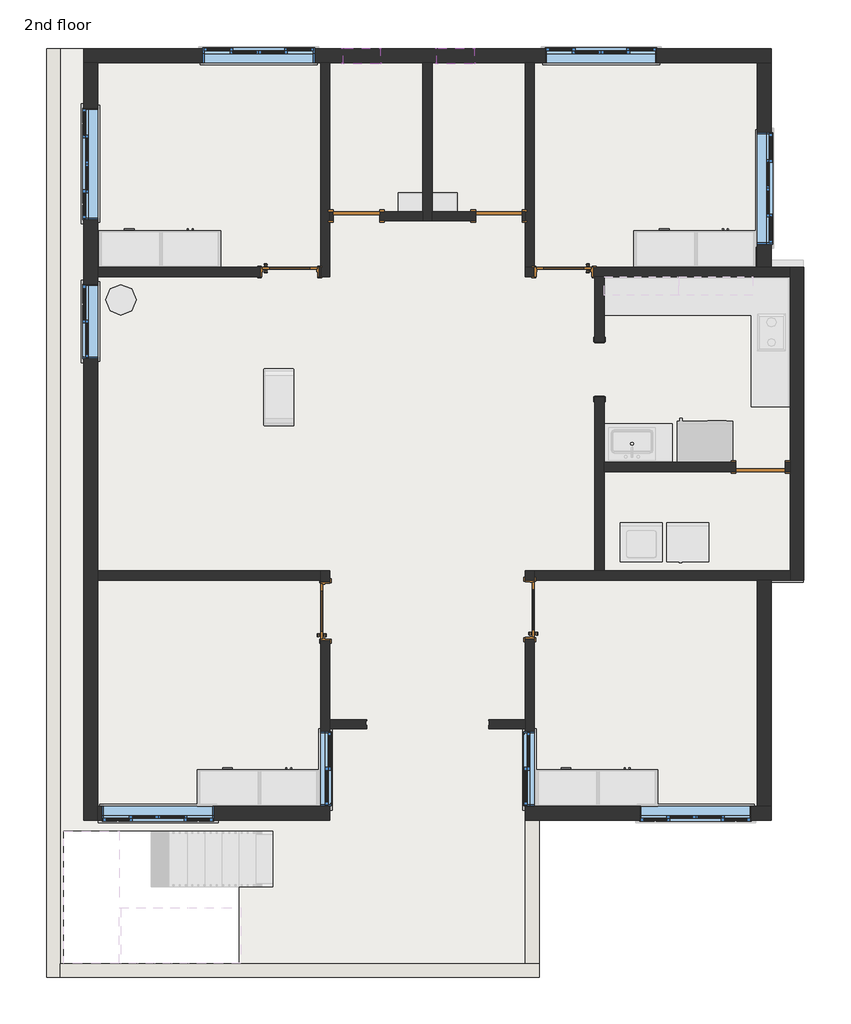
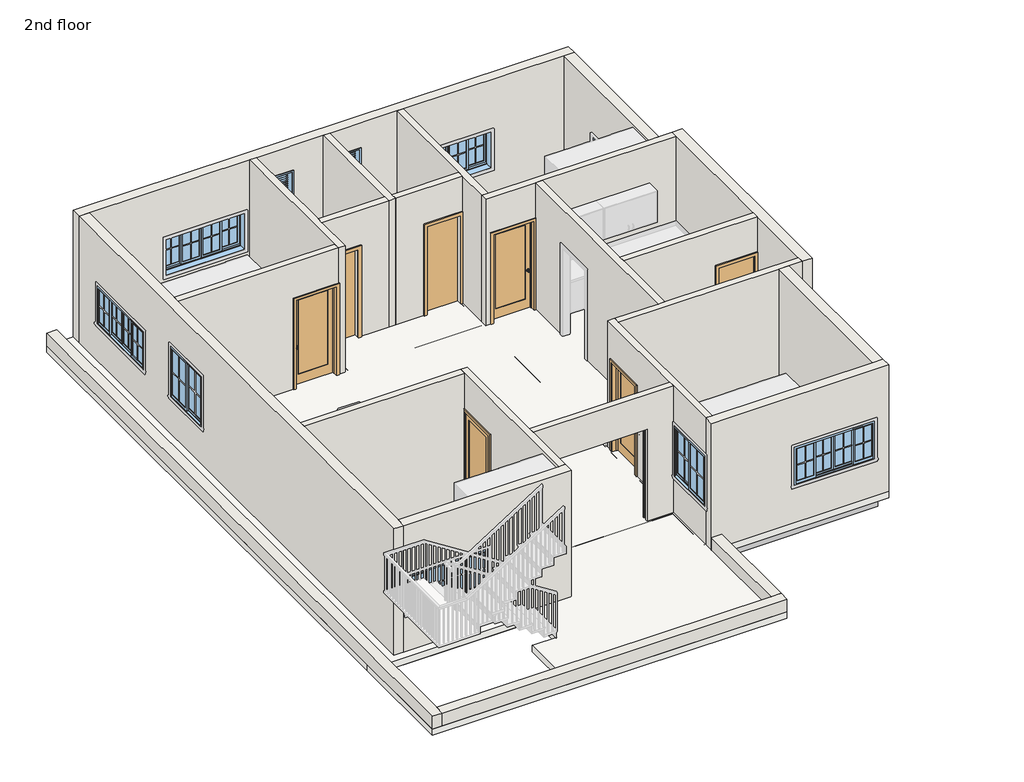
# One storey, part 1 of 4: 24 walls, 11 windows, 7 beams, 7 doors, 1 slab.
# Revit data of these elements (continued)
# Element 45 (IfcWindow, "Window-Sliding-Four : 72\" x 36\"") (continued)
#   Interior Wall Closure = 0' - 2 3/4"
#   Frame Extension = 0' - 0 1/4"
#   Exterior Wall Closure = 0' - 1 1/4"
#   Interior Trim Visibility = yes
#   Indicator Visibility = yes
#   Exterior Trim Visibility = yes
#   Phase Created = New Construction
#   Materials on its faces: "Wood - Stained", "Glass", "Clad - White"
# Element 46 (IfcWindow, "Window-Sliding-Four : 72\" x 36\"")
#   Mark = "29"
#   Window Inset = 0' - 0"
#   Interior Wall Closure = 0' - 2 3/4"
#   Frame Extension = 0' - 0 1/4"
#   Exterior Wall Closure = 0' - 1 1/4"
#   Interior Trim Visibility = yes
#   Indicator Visibility = yes
#   Exterior Trim Visibility = yes
#   Phase Created = New Construction
#   Materials on its faces: "Wood - Stained", "Glass", "Clad - White"
# Element 47 (IfcWindow, "Window-Sliding-Four : 72\" x 36\"")
#   Mark = "30"
#   Window Inset = 0' - 0"
#   Interior Wall Closure = 0' - 2 3/4"
#   Frame Extension = 0' - 0 1/4"
#   Exterior Wall Closure = 0' - 1 1/4"
#   Interior Trim Visibility = yes
#   Indicator Visibility = yes
#   Exterior Trim Visibility = yes
#   Phase Created = New Construction
#   Materials on its faces: "Wood - Stained", "Glass", "Clad - White"
# Element 48 (IfcWindow, "Window-Sliding-Four : 72\" x 36\"")
#   Mark = "31"
#   Window Inset = 0' - 0"
#   Interior Wall Closure = 0' - 2 3/4"
#   Frame Extension = 0' - 0 1/4"
#   Exterior Wall Closure = 0' - 1 1/4"
#   Interior Trim Visibility = yes
#   Indicator Visibility = yes
#   Exterior Trim Visibility = yes
#   Phase Created = New Construction
#   Materials on its faces: "Wood - Stained", "Glass", "Clad - White"
# Element 49 (IfcWindow, "Window-Sliding-Four : 72\" x 36\"")
#   Mark = "35"
#   Window Inset = 0' - 0"
#   Interior Wall Closure = 0' - 2 3/4"
#   Frame Extension = 0' - 0 1/4"
#   Exterior Wall Closure = 0' - 1 1/4"
#   Interior Trim Visibility = yes
#   Indicator Visibility = yes
#   Exterior Trim Visibility = yes
#   Phase Created = New Construction
#   Materials on its faces: "Wood - Stained", "Glass", "Clad - White"
# Element 50 (IfcWindow, "Window-Sliding-Four : 72\" x 36\"")
#   Mark = "36"
#   Window Inset = 0' - 0"
#   Interior Wall Closure = 0' - 2 3/4"
#   Frame Extension = 0' - 0 1/4"
#   Exterior Wall Closure = 0' - 1 1/4"
#   Interior Trim Visibility = yes
#   Indicator Visibility = yes
#   Exterior Trim Visibility = yes
#   Phase Created = New Construction
#   Materials on its faces: "Wood - Stained", "Glass", "Clad - White"
# Materials
#   "Concrete, Cast-in-Place gray": class "Concrete", colour RGB 192 192 192, transparency 0, Description = "Cast-in-place concrete", Cost = 0
#   "Cherry": class "Wood", colour RGB 226 177 128, transparency 0, Description = "Prunus Serotina", Cost = 0
#   "Aluminum": class "Metal", colour RGB 247 247 247, transparency 0, Description = "Aluminum 6061", Cost = 0
#   "Door - Panel": class "Wood", colour RGB 210 159 95, transparency 0, Cost = 0
#   "Door - Frame": colour RGB 118 70 51, transparency 0, Cost = 0
#   "Birch": class "Wood", colour RGB 224 178 126, transparency 0, Description = "Betula Alleghaniensis", Cost = 0
#   "Wood - Stained": class "Wood", colour RGB 224 178 126, transparency 0, Cost = 0
#   "Glass": class "Glass", colour RGB 0 128 192, transparency 0.75, Description = "Soda Lime Glass", Cost = 0
#   "Clad - White": class "Wood", colour RGB 242 242 238, transparency 0, Cost = 0
#   "Default Floor": colour RGB 128 128 128, transparency 0, Cost = 0
#   "Default Wall": colour RGB 128 128 128, transparency 0, Cost = 0
